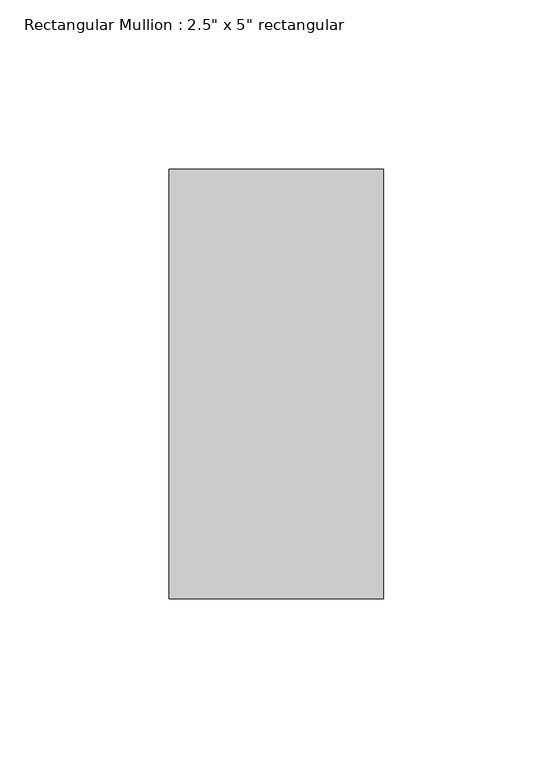
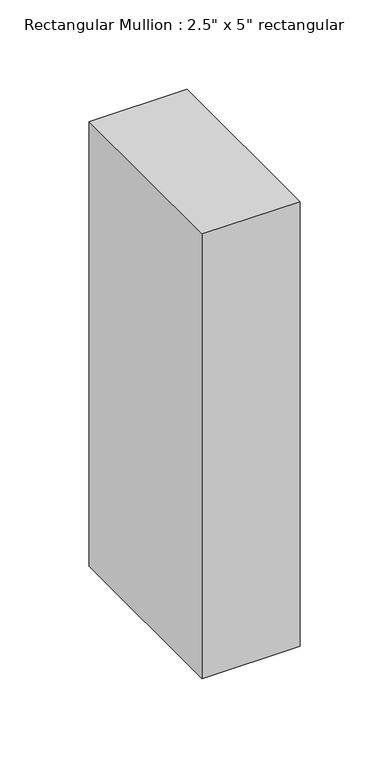
"""IFC4 building model written with IfcOpenShell, lengths in millimetres: member geometry."""

from ifc_helpers import new_model, si_unit, frame, origin, place, context, project, spatial, polyline, outline, extrude, source, transform, mapped, element, save


def member_75d1e245(model_context):
    return source(origin(), model_context, "Body", "SweptSolid", [
        extrude(outline(polyline([(31.75, 63.5), (31.75, -63.5), (-31.75, -63.5), (-31.75, 63.5), (31.75, 63.5)])), frame((0.0, 0.0, -304.8), z_axis=(0.0, 0.0, 1.0), x_axis=(1.0, 0.0, 0.0)), (0.0, 0.0, 1.0), 304.8),
    ])


if __name__ == "__main__":
    model = new_model("IFC4")
    model_context = context("Model", 3, world=origin())
    ifc_project = project(units=[si_unit("LENGTHUNIT", "METRE", prefix="MILLI")], contexts=[model_context])
    site = spatial("IfcSite", under=ifc_project)
    building = spatial("IfcBuilding", under=site)
    placement = place(None, origin())
    member_shape = member_75d1e245(model_context)
    element("IfcMember", 1, ObjectType="Rectangular Mullion : 2.5\" x 5\" rectangular", at=placement, inside=building, context=model_context, shape_type="MappedRepresentation", body=[
        mapped(member_shape, transform((0.0, 0.0, 0.0), x_axis=(1.0, 0.0, 0.0), y_axis=(0.0, 1.0, 0.0), z_axis=(0.0, 0.0, 1.0))),
    ])
    save(model, "model.ifc")

# Revit data of these elements
# Type "Rectangular Mullion : 2.5\" x 5\" rectangular"
#   built-in parameter 1007304 = 0.416667 (stored number, unit not read)
#   built-in parameter 1007301 = 0.104167 (stored number, unit not read)
#   built-in parameter 1007300 = 0.104167 (stored number, unit not read)
# Element 1 (IfcMember, "Rectangular Mullion : 2.5\" x 5\" rectangular")
#   Materials on its faces: "Iron, Ductile"
# Materials
#   "Iron, Ductile": class "Metal", colour RGB 0 0 0, transparency 0, Description = "Ductile cast iron", Cost = 0
